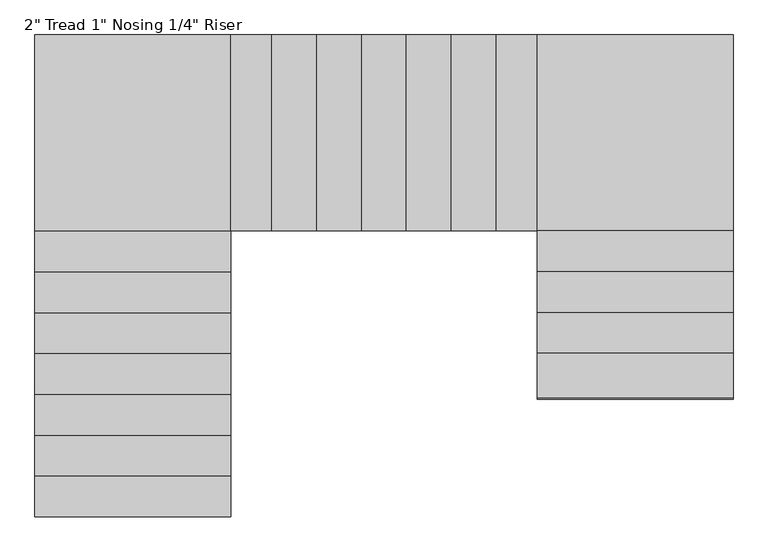
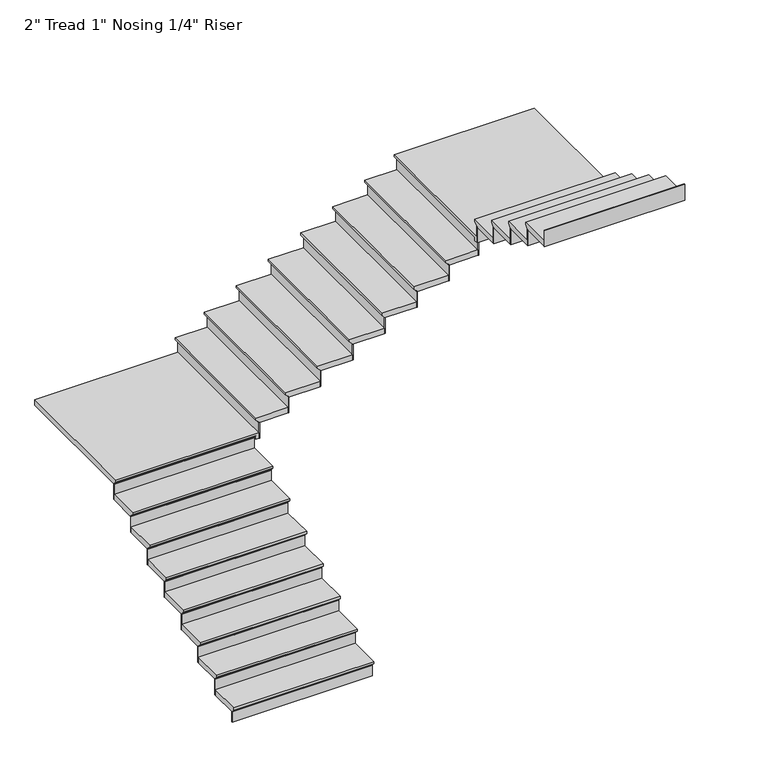
"""IFC4 building model written with IfcOpenShell, lengths in millimetres: stair flight geometry."""

from ifc_helpers import new_model, si_unit, origin, place, context, project, spatial, faceted_brep, source, transform, mapped, element, save


def stair_flight_2ad91a83(model_context):
    return source(origin(), model_context, "Body", "Brep", [
        faceted_brep([(-62544.6636189, 6754.3199577, 126.0928571), (-62544.6636189, 6754.3199577, 145.1428571), (-63763.8636189, 6754.3199577, 145.1428571), (-63763.8636189, 6754.3199577, 126.0928571), (-62544.6636189, 6779.7199577, 100.6928571), (-63763.8636189, 6779.7199577, 100.6928571), (-62544.6636189, 7033.7199577, 145.1428571), (-63763.8636189, 7033.7199577, 145.1428571), (-63763.8636189, 6779.7199577, 94.3428571), (-63763.8636189, 7033.7199577, 94.3428571), (-62544.6636189, 7033.7199577, 94.3428571), (-62544.6636189, 6779.7199577, 94.3428571)], [[[0, 1, 2, 3]], [[4, 0, 3, 5]], [[2, 1, 6, 7]], [[8, 9, 10, 11]], [[2, 7, 9, 8, 5, 3]], [[8, 11, 4, 5]], [[6, 1, 0, 4, 11, 10]], [[7, 6, 10, 9]]]),
        faceted_brep([(-62544.6636189, 6779.7199577, 94.3428571), (-62544.6636189, 6779.7199577, 0.0), (-62544.6636189, 6786.0699577, 0.0), (-62544.6636189, 6786.0699577, 94.3428571), (-63763.8636189, 6779.7199577, 94.3428571), (-63763.8636189, 6786.0699577, 94.3428571), (-63763.8636189, 6786.0699577, 0.0), (-63763.8636189, 6779.7199577, 0.0)], [[[0, 1, 2, 3]], [[4, 5, 6, 7]], [[1, 0, 4, 7]], [[2, 1, 7, 6]], [[3, 2, 6, 5]], [[0, 3, 5, 4]]]),
        faceted_brep([(-62544.6636189, 7033.7199577, 239.4857143), (-62544.6636189, 7033.7199577, 94.3428571), (-62544.6636189, 7040.0699577, 94.3428571), (-62544.6636189, 7040.0699577, 239.4857143), (-63763.8636189, 7033.7199577, 239.4857143), (-63763.8636189, 7040.0699577, 239.4857143), (-63763.8636189, 7040.0699577, 94.3428571), (-63763.8636189, 7033.7199577, 94.3428571)], [[[0, 1, 2, 3]], [[4, 5, 6, 7]], [[1, 0, 4, 7]], [[2, 1, 7, 6]], [[3, 2, 6, 5]], [[0, 3, 5, 4]]]),
        faceted_brep([(-63763.8636189, 7008.3199577, 290.2857143), (-62544.6636189, 7008.3199577, 290.2857143), (-62544.6636189, 7287.7199577, 290.2857143), (-63763.8636189, 7287.7199577, 290.2857143), (-63763.8636189, 7033.7199577, 239.4857143), (-63763.8636189, 7287.7199577, 239.4857143), (-62544.6636189, 7287.7199577, 239.4857143), (-62544.6636189, 7033.7199577, 239.4857143), (-63763.8636189, 7033.7199577, 245.8357143), (-63763.8636189, 7008.3199577, 271.2357143), (-62544.6636189, 7033.7199577, 245.8357143), (-62544.6636189, 7008.3199577, 271.2357143)], [[[0, 1, 2, 3]], [[4, 5, 6, 7]], [[0, 3, 5, 4, 8, 9]], [[4, 7, 10, 8]], [[2, 1, 11, 10, 7, 6]], [[3, 2, 6, 5]], [[11, 1, 0, 9]], [[10, 11, 9, 8]]]),
        faceted_brep([(-62544.6636189, 7287.7199577, 384.6285714), (-62544.6636189, 7287.7199577, 239.4857143), (-62544.6636189, 7294.0699577, 239.4857143), (-62544.6636189, 7294.0699577, 384.6285714), (-63763.8636189, 7287.7199577, 384.6285714), (-63763.8636189, 7294.0699577, 384.6285714), (-63763.8636189, 7294.0699577, 239.4857143), (-63763.8636189, 7287.7199577, 239.4857143)], [[[0, 1, 2, 3]], [[4, 5, 6, 7]], [[1, 0, 4, 7]], [[2, 1, 7, 6]], [[3, 2, 6, 5]], [[0, 3, 5, 4]]]),
        faceted_brep([(-63763.8636189, 7262.3199577, 435.4285714), (-62544.6636189, 7262.3199577, 435.4285714), (-62544.6636189, 7541.7199577, 435.4285714), (-63763.8636189, 7541.7199577, 435.4285714), (-63763.8636189, 7287.7199577, 384.6285714), (-63763.8636189, 7541.7199577, 384.6285714), (-62544.6636189, 7541.7199577, 384.6285714), (-62544.6636189, 7287.7199577, 384.6285714), (-63763.8636189, 7287.7199577, 390.9785714), (-63763.8636189, 7262.3199577, 416.3785714), (-62544.6636189, 7287.7199577, 390.9785714), (-62544.6636189, 7262.3199577, 416.3785714)], [[[0, 1, 2, 3]], [[4, 5, 6, 7]], [[0, 3, 5, 4, 8, 9]], [[4, 7, 10, 8]], [[2, 1, 11, 10, 7, 6]], [[3, 2, 6, 5]], [[11, 1, 0, 9]], [[10, 11, 9, 8]]]),
        faceted_brep([(-62544.6636189, 7541.7199577, 529.7714286), (-62544.6636189, 7541.7199577, 384.6285714), (-62544.6636189, 7548.0699577, 384.6285714), (-62544.6636189, 7548.0699577, 529.7714286), (-63763.8636189, 7541.7199577, 529.7714286), (-63763.8636189, 7548.0699577, 529.7714286), (-63763.8636189, 7548.0699577, 384.6285714), (-63763.8636189, 7541.7199577, 384.6285714)], [[[0, 1, 2, 3]], [[4, 5, 6, 7]], [[1, 0, 4, 7]], [[2, 1, 7, 6]], [[3, 2, 6, 5]], [[0, 3, 5, 4]]]),
        faceted_brep([(-63763.8636189, 7516.3199577, 580.5714286), (-62544.6636189, 7516.3199577, 580.5714286), (-62544.6636189, 7795.7199577, 580.5714286), (-63763.8636189, 7795.7199577, 580.5714286), (-63763.8636189, 7541.7199577, 529.7714286), (-63763.8636189, 7795.7199577, 529.7714286), (-62544.6636189, 7795.7199577, 529.7714286), (-62544.6636189, 7541.7199577, 529.7714286), (-63763.8636189, 7541.7199577, 536.1214286), (-63763.8636189, 7516.3199577, 561.5214286), (-62544.6636189, 7541.7199577, 536.1214286), (-62544.6636189, 7516.3199577, 561.5214286)], [[[0, 1, 2, 3]], [[4, 5, 6, 7]], [[0, 3, 5, 4, 8, 9]], [[4, 7, 10, 8]], [[2, 1, 11, 10, 7, 6]], [[3, 2, 6, 5]], [[11, 1, 0, 9]], [[10, 11, 9, 8]]]),
        faceted_brep([(-62544.6636189, 7795.7199577, 674.9142857), (-62544.6636189, 7795.7199577, 529.7714286), (-62544.6636189, 7802.0699577, 529.7714286), (-62544.6636189, 7802.0699577, 674.9142857), (-63763.8636189, 7795.7199577, 674.9142857), (-63763.8636189, 7802.0699577, 674.9142857), (-63763.8636189, 7802.0699577, 529.7714286), (-63763.8636189, 7795.7199577, 529.7714286)], [[[0, 1, 2, 3]], [[4, 5, 6, 7]], [[1, 0, 4, 7]], [[2, 1, 7, 6]], [[3, 2, 6, 5]], [[0, 3, 5, 4]]]),
        faceted_brep([(-63763.8636189, 7770.3199577, 725.7142857), (-62544.6636189, 7770.3199577, 725.7142857), (-62544.6636189, 8049.7199577, 725.7142857), (-63763.8636189, 8049.7199577, 725.7142857), (-63763.8636189, 7795.7199577, 674.9142857), (-63763.8636189, 8049.7199577, 674.9142857), (-62544.6636189, 8049.7199577, 674.9142857), (-62544.6636189, 7795.7199577, 674.9142857), (-63763.8636189, 7795.7199577, 681.2642857), (-63763.8636189, 7770.3199577, 706.6642857), (-62544.6636189, 7795.7199577, 681.2642857), (-62544.6636189, 7770.3199577, 706.6642857)], [[[0, 1, 2, 3]], [[4, 5, 6, 7]], [[0, 3, 5, 4, 8, 9]], [[4, 7, 10, 8]], [[2, 1, 11, 10, 7, 6]], [[3, 2, 6, 5]], [[11, 1, 0, 9]], [[10, 11, 9, 8]]]),
        faceted_brep([(-62544.6636189, 8049.7199577, 820.0571429), (-62544.6636189, 8049.7199577, 674.9142857), (-62544.6636189, 8056.0699577, 674.9142857), (-62544.6636189, 8056.0699577, 820.0571429), (-63763.8636189, 8049.7199577, 820.0571429), (-63763.8636189, 8056.0699577, 820.0571429), (-63763.8636189, 8056.0699577, 674.9142857), (-63763.8636189, 8049.7199577, 674.9142857)], [[[0, 1, 2, 3]], [[4, 5, 6, 7]], [[1, 0, 4, 7]], [[2, 1, 7, 6]], [[3, 2, 6, 5]], [[0, 3, 5, 4]]]),
        faceted_brep([(-63763.8636189, 8024.3199577, 870.8571429), (-62544.6636189, 8024.3199577, 870.8571429), (-62544.6636189, 8303.7199577, 870.8571429), (-63763.8636189, 8303.7199577, 870.8571429), (-63763.8636189, 8049.7199577, 820.0571429), (-63763.8636189, 8303.7199577, 820.0571429), (-62544.6636189, 8303.7199577, 820.0571429), (-62544.6636189, 8049.7199577, 820.0571429), (-63763.8636189, 8049.7199577, 826.4071429), (-63763.8636189, 8024.3199577, 851.8071429), (-62544.6636189, 8049.7199577, 826.4071429), (-62544.6636189, 8024.3199577, 851.8071429)], [[[0, 1, 2, 3]], [[4, 5, 6, 7]], [[0, 3, 5, 4, 8, 9]], [[4, 7, 10, 8]], [[2, 1, 11, 10, 7, 6]], [[3, 2, 6, 5]], [[11, 1, 0, 9]], [[10, 11, 9, 8]]]),
        faceted_brep([(-62544.6636189, 8303.7199577, 965.2), (-62544.6636189, 8303.7199577, 820.0571429), (-62544.6636189, 8310.0699577, 820.0571429), (-62544.6636189, 8310.0699577, 965.2), (-63763.8636189, 8303.7199577, 965.2), (-63763.8636189, 8310.0699577, 965.2), (-63763.8636189, 8310.0699577, 820.0571429), (-63763.8636189, 8303.7199577, 820.0571429)], [[[0, 1, 2, 3]], [[4, 5, 6, 7]], [[1, 0, 4, 7]], [[2, 1, 7, 6]], [[3, 2, 6, 5]], [[0, 3, 5, 4]]]),
        faceted_brep([(-63763.8636189, 8278.3199577, 1016.0), (-62544.6636189, 8278.3199577, 1016.0), (-62544.6636189, 8557.7199577, 1016.0), (-63763.8636189, 8557.7199577, 1016.0), (-63763.8636189, 8303.7199577, 965.2), (-63763.8636189, 8557.7199577, 965.2), (-62544.6636189, 8557.7199577, 965.2), (-62544.6636189, 8303.7199577, 965.2), (-63763.8636189, 8303.7199577, 971.55), (-63763.8636189, 8278.3199577, 996.95), (-62544.6636189, 8303.7199577, 971.55), (-62544.6636189, 8278.3199577, 996.95)], [[[0, 1, 2, 3]], [[4, 5, 6, 7]], [[0, 3, 5, 4, 8, 9]], [[4, 7, 10, 8]], [[2, 1, 11, 10, 7, 6]], [[3, 2, 6, 5]], [[11, 1, 0, 9]], [[10, 11, 9, 8]]]),
        faceted_brep([(-62544.6636189, 8557.7199577, 1110.3428571), (-62544.6636189, 8557.7199577, 965.2), (-62544.6636189, 8564.0699577, 965.2), (-62544.6636189, 8564.0699577, 1110.3428571), (-63763.8636189, 8557.7199577, 1110.3428571), (-63763.8636189, 8564.0699577, 1110.3428571), (-63763.8636189, 8564.0699577, 965.2), (-63763.8636189, 8557.7199577, 965.2)], [[[0, 1, 2, 3]], [[4, 5, 6, 7]], [[1, 0, 4, 7]], [[2, 1, 7, 6]], [[3, 2, 6, 5]], [[0, 3, 5, 4]]]),
        faceted_brep([(-62519.2636189, 9751.5199577, 1161.1428571), (-63763.8636189, 9751.5199577, 1161.1428571), (-63763.8636189, 8532.3199577, 1161.1428571), (-62519.2636189, 8532.3199577, 1161.1428571), (-63763.8636189, 9751.5199577, 1110.3428571), (-62519.2636189, 9751.5199577, 1110.3428571), (-62519.2636189, 8532.3199577, 1110.3428571), (-62544.6636189, 8532.3199577, 1110.3428571), (-62544.6636189, 8557.7199577, 1110.3428571), (-63763.8636189, 8557.7199577, 1110.3428571), (-63763.8636189, 8557.7199577, 1116.6928571), (-63763.8636189, 8532.3199577, 1142.0928571), (-62544.6636189, 8557.7199577, 1116.6928571), (-62544.6636189, 8532.3199577, 1142.0928571)], [[[0, 1, 2, 3]], [[4, 5, 6, 7, 8, 9]], [[1, 0, 5, 4]], [[2, 1, 4, 9, 10, 11]], [[9, 8, 12, 10]], [[8, 7, 13, 12]], [[3, 2, 11, 13, 7, 6]], [[0, 3, 6, 5]], [[11, 10, 12, 13]]]),
        faceted_brep([(-62519.2636189, 8532.3199577, 1255.4857143), (-62519.2636189, 8532.3199577, 1110.3428571), (-62512.9136189, 8532.3199577, 1110.3428571), (-62512.9136189, 8532.3199577, 1255.4857143), (-62519.2636189, 9751.5199577, 1255.4857143), (-62512.9136189, 9751.5199577, 1255.4857143), (-62512.9136189, 9751.5199577, 1110.3428571), (-62519.2636189, 9751.5199577, 1110.3428571)], [[[0, 1, 2, 3]], [[4, 5, 6, 7]], [[1, 0, 4, 7]], [[2, 1, 7, 6]], [[3, 2, 6, 5]], [[0, 3, 5, 4]]]),
        faceted_brep([(-62544.6636189, 9751.5199577, 1306.2857143), (-62544.6636189, 8532.3199577, 1306.2857143), (-62265.2636189, 8532.3199577, 1306.2857143), (-62265.2636189, 9751.5199577, 1306.2857143), (-62519.2636189, 9751.5199577, 1255.4857143), (-62265.2636189, 9751.5199577, 1255.4857143), (-62265.2636189, 8532.3199577, 1255.4857143), (-62519.2636189, 8532.3199577, 1255.4857143), (-62519.2636189, 9751.5199577, 1261.8357143), (-62544.6636189, 9751.5199577, 1287.2357143), (-62519.2636189, 8532.3199577, 1261.8357143), (-62544.6636189, 8532.3199577, 1287.2357143)], [[[0, 1, 2, 3]], [[4, 5, 6, 7]], [[0, 3, 5, 4, 8, 9]], [[4, 7, 10, 8]], [[2, 1, 11, 10, 7, 6]], [[3, 2, 6, 5]], [[11, 1, 0, 9]], [[10, 11, 9, 8]]]),
        faceted_brep([(-62265.2636189, 8532.3199577, 1400.6285714), (-62265.2636189, 8532.3199577, 1255.4857143), (-62258.9136189, 8532.3199577, 1255.4857143), (-62258.9136189, 8532.3199577, 1400.6285714), (-62265.2636189, 9751.5199577, 1400.6285714), (-62258.9136189, 9751.5199577, 1400.6285714), (-62258.9136189, 9751.5199577, 1255.4857143), (-62265.2636189, 9751.5199577, 1255.4857143)], [[[0, 1, 2, 3]], [[4, 5, 6, 7]], [[1, 0, 4, 7]], [[2, 1, 7, 6]], [[3, 2, 6, 5]], [[0, 3, 5, 4]]]),
        faceted_brep([(-62290.6636189, 9751.5199577, 1451.4285714), (-62290.6636189, 8532.3199577, 1451.4285714), (-61985.8636189, 8532.3199577, 1451.4285714), (-61985.8636189, 9751.5199577, 1451.4285714), (-62265.2636189, 9751.5199577, 1400.6285714), (-61985.8636189, 9751.5199577, 1400.6285714), (-61985.8636189, 8532.3199577, 1400.6285714), (-62265.2636189, 8532.3199577, 1400.6285714), (-62265.2636189, 9751.5199577, 1406.9785714), (-62290.6636189, 9751.5199577, 1432.3785714), (-62265.2636189, 8532.3199577, 1406.9785714), (-62290.6636189, 8532.3199577, 1432.3785714)], [[[0, 1, 2, 3]], [[4, 5, 6, 7]], [[0, 3, 5, 4, 8, 9]], [[4, 7, 10, 8]], [[2, 1, 11, 10, 7, 6]], [[3, 2, 6, 5]], [[11, 1, 0, 9]], [[10, 11, 9, 8]]]),
        faceted_brep([(-61985.8636189, 8532.3199577, 1545.7714286), (-61985.8636189, 8532.3199577, 1400.6285714), (-61979.5136189, 8532.3199577, 1400.6285714), (-61979.5136189, 8532.3199577, 1545.7714286), (-61985.8636189, 9751.5199577, 1545.7714286), (-61979.5136189, 9751.5199577, 1545.7714286), (-61979.5136189, 9751.5199577, 1400.6285714), (-61985.8636189, 9751.5199577, 1400.6285714)], [[[0, 1, 2, 3]], [[4, 5, 6, 7]], [[1, 0, 4, 7]], [[2, 1, 7, 6]], [[3, 2, 6, 5]], [[0, 3, 5, 4]]]),
        faceted_brep([(-62011.2636189, 9751.5199577, 1596.5714286), (-62011.2636189, 8532.3199577, 1596.5714286), (-61706.4636189, 8532.3199577, 1596.5714286), (-61706.4636189, 9751.5199577, 1596.5714286), (-61985.8636189, 9751.5199577, 1545.7714286), (-61706.4636189, 9751.5199577, 1545.7714286), (-61706.4636189, 8532.3199577, 1545.7714286), (-61985.8636189, 8532.3199577, 1545.7714286), (-61985.8636189, 9751.5199577, 1552.1214286), (-62011.2636189, 9751.5199577, 1577.5214286), (-61985.8636189, 8532.3199577, 1552.1214286), (-62011.2636189, 8532.3199577, 1577.5214286)], [[[0, 1, 2, 3]], [[4, 5, 6, 7]], [[0, 3, 5, 4, 8, 9]], [[4, 7, 10, 8]], [[2, 1, 11, 10, 7, 6]], [[3, 2, 6, 5]], [[11, 1, 0, 9]], [[10, 11, 9, 8]]]),
        faceted_brep([(-61706.4636189, 8532.3199577, 1690.9142857), (-61706.4636189, 8532.3199577, 1545.7714286), (-61700.1136189, 8532.3199577, 1545.7714286), (-61700.1136189, 8532.3199577, 1690.9142857), (-61706.4636189, 9751.5199577, 1690.9142857), (-61700.1136189, 9751.5199577, 1690.9142857), (-61700.1136189, 9751.5199577, 1545.7714286), (-61706.4636189, 9751.5199577, 1545.7714286)], [[[0, 1, 2, 3]], [[4, 5, 6, 7]], [[1, 0, 4, 7]], [[2, 1, 7, 6]], [[3, 2, 6, 5]], [[0, 3, 5, 4]]]),
        faceted_brep([(-61731.8636189, 9751.5199577, 1741.7142857), (-61731.8636189, 8532.3199577, 1741.7142857), (-61427.0636189, 8532.3199577, 1741.7142857), (-61427.0636189, 9751.5199577, 1741.7142857), (-61706.4636189, 9751.5199577, 1690.9142857), (-61427.0636189, 9751.5199577, 1690.9142857), (-61427.0636189, 8532.3199577, 1690.9142857), (-61706.4636189, 8532.3199577, 1690.9142857), (-61706.4636189, 9751.5199577, 1697.2642857), (-61731.8636189, 9751.5199577, 1722.6642857), (-61706.4636189, 8532.3199577, 1697.2642857), (-61731.8636189, 8532.3199577, 1722.6642857)], [[[0, 1, 2, 3]], [[4, 5, 6, 7]], [[0, 3, 5, 4, 8, 9]], [[4, 7, 10, 8]], [[2, 1, 11, 10, 7, 6]], [[3, 2, 6, 5]], [[11, 1, 0, 9]], [[10, 11, 9, 8]]]),
        faceted_brep([(-61427.0636189, 8532.3199577, 1836.0571429), (-61427.0636189, 8532.3199577, 1690.9142857), (-61420.7136189, 8532.3199577, 1690.9142857), (-61420.7136189, 8532.3199577, 1836.0571429), (-61427.0636189, 9751.5199577, 1836.0571429), (-61420.7136189, 9751.5199577, 1836.0571429), (-61420.7136189, 9751.5199577, 1690.9142857), (-61427.0636189, 9751.5199577, 1690.9142857)], [[[0, 1, 2, 3]], [[4, 5, 6, 7]], [[1, 0, 4, 7]], [[2, 1, 7, 6]], [[3, 2, 6, 5]], [[0, 3, 5, 4]]]),
        faceted_brep([(-61452.4636189, 9751.5199577, 1886.8571429), (-61452.4636189, 8532.3199577, 1886.8571429), (-61147.6636189, 8532.3199577, 1886.8571429), (-61147.6636189, 9751.5199577, 1886.8571429), (-61427.0636189, 9751.5199577, 1836.0571429), (-61147.6636189, 9751.5199577, 1836.0571429), (-61147.6636189, 8532.3199577, 1836.0571429), (-61427.0636189, 8532.3199577, 1836.0571429), (-61427.0636189, 9751.5199577, 1842.4071429), (-61452.4636189, 9751.5199577, 1867.8071429), (-61427.0636189, 8532.3199577, 1842.4071429), (-61452.4636189, 8532.3199577, 1867.8071429)], [[[0, 1, 2, 3]], [[4, 5, 6, 7]], [[0, 3, 5, 4, 8, 9]], [[4, 7, 10, 8]], [[2, 1, 11, 10, 7, 6]], [[3, 2, 6, 5]], [[11, 1, 0, 9]], [[10, 11, 9, 8]]]),
        faceted_brep([(-61147.6636189, 8532.3199577, 1981.2), (-61147.6636189, 8532.3199577, 1836.0571429), (-61141.3136189, 8532.3199577, 1836.0571429), (-61141.3136189, 8532.3199577, 1981.2), (-61147.6636189, 9751.5199577, 1981.2), (-61141.3136189, 9751.5199577, 1981.2), (-61141.3136189, 9751.5199577, 1836.0571429), (-61147.6636189, 9751.5199577, 1836.0571429)], [[[0, 1, 2, 3]], [[4, 5, 6, 7]], [[1, 0, 4, 7]], [[2, 1, 7, 6]], [[3, 2, 6, 5]], [[0, 3, 5, 4]]]),
        faceted_brep([(-61173.0636189, 9751.5199577, 2032.0), (-61173.0636189, 8532.3199577, 2032.0), (-60868.2636189, 8532.3199577, 2032.0), (-60868.2636189, 9751.5199577, 2032.0), (-61147.6636189, 9751.5199577, 1981.2), (-60868.2636189, 9751.5199577, 1981.2), (-60868.2636189, 8532.3199577, 1981.2), (-61147.6636189, 8532.3199577, 1981.2), (-61147.6636189, 9751.5199577, 1987.55), (-61173.0636189, 9751.5199577, 2012.95), (-61147.6636189, 8532.3199577, 1987.55), (-61173.0636189, 8532.3199577, 2012.95)], [[[0, 1, 2, 3]], [[4, 5, 6, 7]], [[0, 3, 5, 4, 8, 9]], [[4, 7, 10, 8]], [[2, 1, 11, 10, 7, 6]], [[3, 2, 6, 5]], [[11, 1, 0, 9]], [[10, 11, 9, 8]]]),
        faceted_brep([(-60868.2636189, 8532.3199577, 2126.3428571), (-60868.2636189, 8532.3199577, 1981.2), (-60861.9136189, 8532.3199577, 1981.2), (-60861.9136189, 8532.3199577, 2126.3428571), (-60868.2636189, 9751.5199577, 2126.3428571), (-60861.9136189, 9751.5199577, 2126.3428571), (-60861.9136189, 9751.5199577, 1981.2), (-60868.2636189, 9751.5199577, 1981.2)], [[[0, 1, 2, 3]], [[4, 5, 6, 7]], [[1, 0, 4, 7]], [[2, 1, 7, 6]], [[3, 2, 6, 5]], [[0, 3, 5, 4]]]),
        faceted_brep([(-60893.6636189, 9751.5199577, 2177.1428571), (-60893.6636189, 8532.3199577, 2177.1428571), (-60614.2636189, 8532.3199577, 2177.1428571), (-60614.2636189, 9751.5199577, 2177.1428571), (-60868.2636189, 9751.5199577, 2126.3428571), (-60614.2636189, 9751.5199577, 2126.3428571), (-60614.2636189, 8532.3199577, 2126.3428571), (-60868.2636189, 8532.3199577, 2126.3428571), (-60868.2636189, 9751.5199577, 2132.6928571), (-60893.6636189, 9751.5199577, 2158.0928571), (-60868.2636189, 8532.3199577, 2132.6928571), (-60893.6636189, 8532.3199577, 2158.0928571)], [[[0, 1, 2, 3]], [[4, 5, 6, 7]], [[0, 3, 5, 4, 8, 9]], [[4, 7, 10, 8]], [[2, 1, 11, 10, 7, 6]], [[3, 2, 6, 5]], [[11, 1, 0, 9]], [[10, 11, 9, 8]]]),
        faceted_brep([(-60614.2636189, 8532.3199577, 2271.4857143), (-60614.2636189, 8532.3199577, 2126.3428571), (-60607.9136189, 8532.3199577, 2126.3428571), (-60607.9136189, 8532.3199577, 2271.4857143), (-60614.2636189, 9751.5199577, 2271.4857143), (-60607.9136189, 9751.5199577, 2271.4857143), (-60607.9136189, 9751.5199577, 2126.3428571), (-60614.2636189, 9751.5199577, 2126.3428571)], [[[0, 1, 2, 3]], [[4, 5, 6, 7]], [[1, 0, 4, 7]], [[2, 1, 7, 6]], [[3, 2, 6, 5]], [[0, 3, 5, 4]]]),
        faceted_brep([(-59420.4636189, 8506.9199577, 2322.2857143), (-59420.4636189, 9751.5199577, 2322.2857143), (-60639.6636189, 9751.5199577, 2322.2857143), (-60639.6636189, 8506.9199577, 2322.2857143), (-59420.4636189, 9751.5199577, 2271.4857143), (-59420.4636189, 8506.9199577, 2271.4857143), (-60639.6636189, 8506.9199577, 2271.4857143), (-60639.6636189, 8532.3199577, 2271.4857143), (-60614.2636189, 8532.3199577, 2271.4857143), (-60614.2636189, 9751.5199577, 2271.4857143), (-60614.2636189, 9751.5199577, 2277.8357143), (-60639.6636189, 9751.5199577, 2303.2357143), (-60614.2636189, 8532.3199577, 2277.8357143), (-60639.6636189, 8532.3199577, 2303.2357143)], [[[0, 1, 2, 3]], [[4, 5, 6, 7, 8, 9]], [[1, 0, 5, 4]], [[2, 1, 4, 9, 10, 11]], [[9, 8, 12, 10]], [[8, 7, 13, 12]], [[3, 2, 11, 13, 7, 6]], [[0, 3, 6, 5]], [[11, 10, 12, 13]]]),
        faceted_brep([(-60639.6636189, 8506.9199577, 2416.6285714), (-60639.6636189, 8506.9199577, 2271.4857143), (-60639.6636189, 8500.5699577, 2271.4857143), (-60639.6636189, 8500.5699577, 2416.6285714), (-59420.4636189, 8506.9199577, 2416.6285714), (-59420.4636189, 8500.5699577, 2416.6285714), (-59420.4636189, 8500.5699577, 2271.4857143), (-59420.4636189, 8506.9199577, 2271.4857143)], [[[0, 1, 2, 3]], [[4, 5, 6, 7]], [[1, 0, 4, 7]], [[2, 1, 7, 6]], [[3, 2, 6, 5]], [[0, 3, 5, 4]]]),
        faceted_brep([(-59420.4636189, 8532.3199577, 2467.4285714), (-60639.6636189, 8532.3199577, 2467.4285714), (-60639.6636189, 8252.9199577, 2467.4285714), (-59420.4636189, 8252.9199577, 2467.4285714), (-59420.4636189, 8506.9199577, 2416.6285714), (-59420.4636189, 8252.9199577, 2416.6285714), (-60639.6636189, 8252.9199577, 2416.6285714), (-60639.6636189, 8506.9199577, 2416.6285714), (-59420.4636189, 8506.9199577, 2422.9785714), (-59420.4636189, 8532.3199577, 2448.3785714), (-60639.6636189, 8506.9199577, 2422.9785714), (-60639.6636189, 8532.3199577, 2448.3785714)], [[[0, 1, 2, 3]], [[4, 5, 6, 7]], [[0, 3, 5, 4, 8, 9]], [[4, 7, 10, 8]], [[2, 1, 11, 10, 7, 6]], [[3, 2, 6, 5]], [[11, 1, 0, 9]], [[10, 11, 9, 8]]]),
        faceted_brep([(-60639.6636189, 8252.9199577, 2561.7714286), (-60639.6636189, 8252.9199577, 2416.6285714), (-60639.6636189, 8246.5699577, 2416.6285714), (-60639.6636189, 8246.5699577, 2561.7714286), (-59420.4636189, 8252.9199577, 2561.7714286), (-59420.4636189, 8246.5699577, 2561.7714286), (-59420.4636189, 8246.5699577, 2416.6285714), (-59420.4636189, 8252.9199577, 2416.6285714)], [[[0, 1, 2, 3]], [[4, 5, 6, 7]], [[1, 0, 4, 7]], [[2, 1, 7, 6]], [[3, 2, 6, 5]], [[0, 3, 5, 4]]]),
        faceted_brep([(-59420.4636189, 8278.3199577, 2612.5714286), (-60639.6636189, 8278.3199577, 2612.5714286), (-60639.6636189, 7998.9199577, 2612.5714286), (-59420.4636189, 7998.9199577, 2612.5714286), (-59420.4636189, 8252.9199577, 2561.7714286), (-59420.4636189, 7998.9199577, 2561.7714286), (-60639.6636189, 7998.9199577, 2561.7714286), (-60639.6636189, 8252.9199577, 2561.7714286), (-59420.4636189, 8252.9199577, 2568.1214286), (-59420.4636189, 8278.3199577, 2593.5214286), (-60639.6636189, 8252.9199577, 2568.1214286), (-60639.6636189, 8278.3199577, 2593.5214286)], [[[0, 1, 2, 3]], [[4, 5, 6, 7]], [[0, 3, 5, 4, 8, 9]], [[4, 7, 10, 8]], [[2, 1, 11, 10, 7, 6]], [[3, 2, 6, 5]], [[11, 1, 0, 9]], [[10, 11, 9, 8]]]),
        faceted_brep([(-60639.6636189, 7998.9199577, 2706.9142857), (-60639.6636189, 7998.9199577, 2561.7714286), (-60639.6636189, 7992.5699577, 2561.7714286), (-60639.6636189, 7992.5699577, 2706.9142857), (-59420.4636189, 7998.9199577, 2706.9142857), (-59420.4636189, 7992.5699577, 2706.9142857), (-59420.4636189, 7992.5699577, 2561.7714286), (-59420.4636189, 7998.9199577, 2561.7714286)], [[[0, 1, 2, 3]], [[4, 5, 6, 7]], [[1, 0, 4, 7]], [[2, 1, 7, 6]], [[3, 2, 6, 5]], [[0, 3, 5, 4]]]),
        faceted_brep([(-59420.4636189, 8024.3199577, 2757.7142857), (-60639.6636189, 8024.3199577, 2757.7142857), (-60639.6636189, 7744.9199577, 2757.7142857), (-59420.4636189, 7744.9199577, 2757.7142857), (-59420.4636189, 7998.9199577, 2706.9142857), (-59420.4636189, 7744.9199577, 2706.9142857), (-60639.6636189, 7744.9199577, 2706.9142857), (-60639.6636189, 7998.9199577, 2706.9142857), (-59420.4636189, 7998.9199577, 2713.2642857), (-59420.4636189, 8024.3199577, 2738.6642857), (-60639.6636189, 7998.9199577, 2713.2642857), (-60639.6636189, 8024.3199577, 2738.6642857)], [[[0, 1, 2, 3]], [[4, 5, 6, 7]], [[0, 3, 5, 4, 8, 9]], [[4, 7, 10, 8]], [[2, 1, 11, 10, 7, 6]], [[3, 2, 6, 5]], [[11, 1, 0, 9]], [[10, 11, 9, 8]]]),
        faceted_brep([(-60639.6636189, 7744.9199577, 2852.0571429), (-60639.6636189, 7744.9199577, 2706.9142857), (-60639.6636189, 7738.5699577, 2706.9142857), (-60639.6636189, 7738.5699577, 2852.0571429), (-59420.4636189, 7744.9199577, 2852.0571429), (-59420.4636189, 7738.5699577, 2852.0571429), (-59420.4636189, 7738.5699577, 2706.9142857), (-59420.4636189, 7744.9199577, 2706.9142857)], [[[0, 1, 2, 3]], [[4, 5, 6, 7]], [[1, 0, 4, 7]], [[2, 1, 7, 6]], [[3, 2, 6, 5]], [[0, 3, 5, 4]]]),
        faceted_brep([(-60639.6636189, 7490.9199577, 2997.2), (-60639.6636189, 7490.9199577, 2852.0571429), (-60639.6636189, 7484.5699577, 2852.0571429), (-60639.6636189, 7484.5699577, 2997.2), (-59420.4636189, 7490.9199577, 2997.2), (-59420.4636189, 7484.5699577, 2997.2), (-59420.4636189, 7484.5699577, 2852.0571429), (-59420.4636189, 7490.9199577, 2852.0571429)], [[[0, 1, 2, 3]], [[4, 5, 6, 7]], [[1, 0, 4, 7]], [[2, 1, 7, 6]], [[3, 2, 6, 5]], [[0, 3, 5, 4]]]),
        faceted_brep([(-59420.4636189, 7770.3199577, 2902.8571429), (-60639.6636189, 7770.3199577, 2902.8571429), (-60639.6636189, 7490.9199577, 2902.8571429), (-59420.4636189, 7490.9199577, 2902.8571429), (-59420.4636189, 7744.9199577, 2852.0571429), (-59420.4636189, 7490.9199577, 2852.0571429), (-60639.6636189, 7490.9199577, 2852.0571429), (-60639.6636189, 7744.9199577, 2852.0571429), (-59420.4636189, 7744.9199577, 2858.4071429), (-59420.4636189, 7770.3199577, 2883.8071429), (-60639.6636189, 7744.9199577, 2858.4071429), (-60639.6636189, 7770.3199577, 2883.8071429)], [[[0, 1, 2, 3]], [[4, 5, 6, 7]], [[0, 3, 5, 4, 8, 9]], [[4, 7, 10, 8]], [[2, 1, 11, 10, 7, 6]], [[3, 2, 6, 5]], [[11, 1, 0, 9]], [[10, 11, 9, 8]]]),
    ])


if __name__ == "__main__":
    model = new_model("IFC4")
    model_context = context("Model", 3, world=origin())
    ifc_project = project(units=[si_unit("LENGTHUNIT", "METRE", prefix="MILLI")], contexts=[model_context])
    site = spatial("IfcSite", under=ifc_project)
    building = spatial("IfcBuilding", under=site)
    placement = place(None, origin())
    stair_flight_shape = stair_flight_2ad91a83(model_context)
    element("IfcStairFlight", 1, ObjectType="2\" Tread 1\" Nosing 1/4\" Riser", at=placement, inside=building, context=model_context, shape_type="MappedRepresentation", body=[
        mapped(stair_flight_shape, transform((0.0, 0.0, 0.0), x_axis=(1.0, 0.0, 0.0), y_axis=(0.0, 1.0, 0.0), z_axis=(0.0, 0.0, 1.0))),
    ])
    save(model, "model.ifc")
